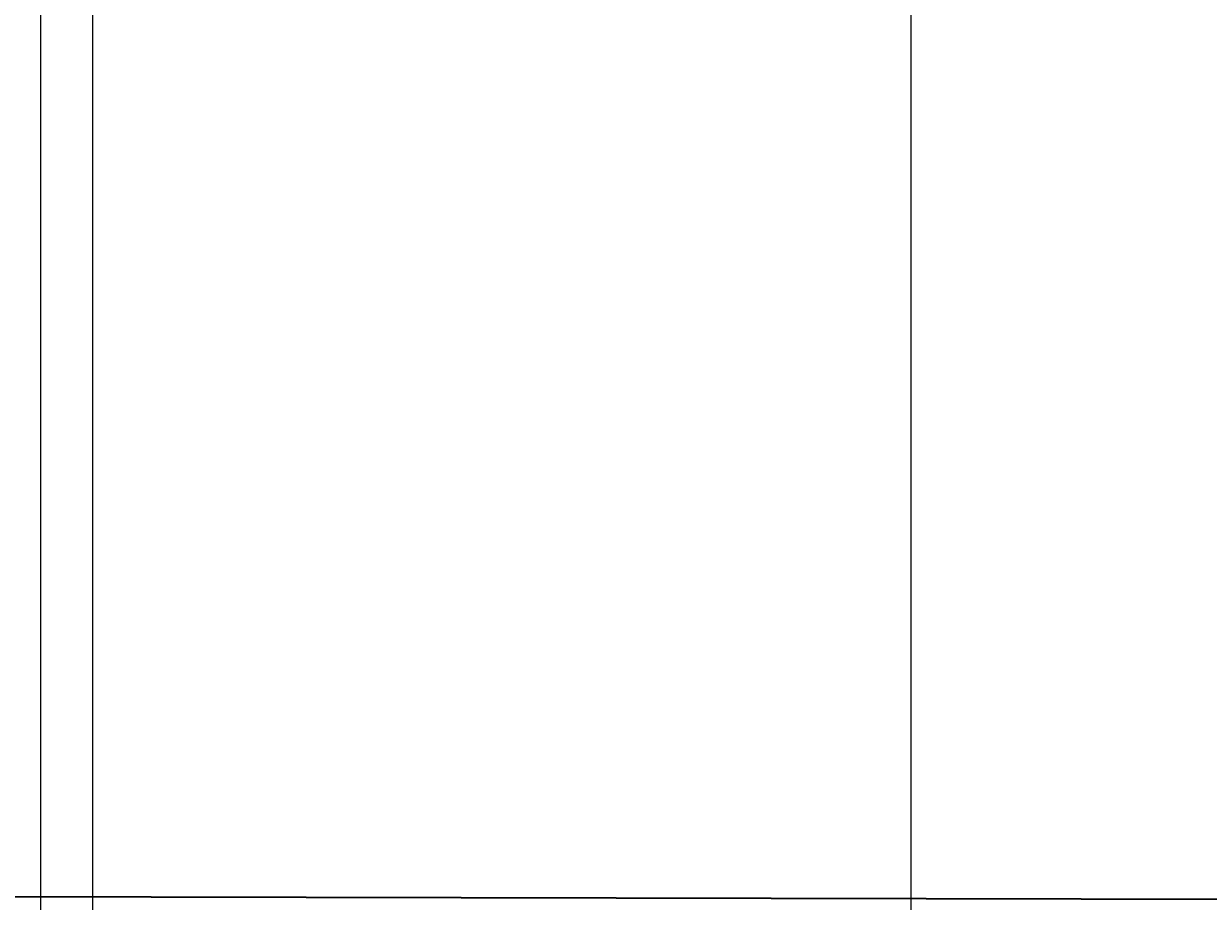
# Model space of a CAD drawing. Units: inches. Extents: x 27 to 200, y -50 to 102.
# Tile 21 of 26: x 145 to 172, y 19 to 39. Entities that reach past the tile are written whole.
import ezdxf

# ---------------------------------------------------------------- set-up
doc = ezdxf.new("R2010")
doc.units = ezdxf.units.IN
doc.header["$MEASUREMENT"] = 0
doc.layers.add('A-ANNO-DIMS', color=2, linetype='Continuous', lineweight=18)
doc.layers.add('A-ELEV', color=7, linetype='Continuous', lineweight=35)
doc.styles.get("Standard").update_dxf_attribs({"font": 'arial.ttf'})
doc.dimstyles.get("Standard").update_dxf_attribs({"dimtxt": 0.18, "dimasz": 0.18, "dimexe": 0.18, "dimexo": 0.0625, "dimgap": 0.09, "dimtad": 0, "dimtih": 1, "dimtoh": 1, "dimdec": 4, "dimzin": 0, "dimdsep": 46, "dimtxsty": 'Standard', "dimcen": 0.09, "dimadec": 0, "dimazin": 0, "dimtfac": 1, "dimtdec": 4, "dimtofl": 0, "dimtmove": 0, "dimatfit": 3, "dimfxl": 1, "dimtolj": 1, "dimtzin": 0, "dimarcsym": 0})

# ---------------------------------------------------------------- blocks, each defined once
blk = doc.blocks.new('*D48')
at = {"layer": 'A-ANNO-DIMS', "color": 0, "lineweight": -2, "transparency": 16777216}
for p, q in [((84.479, 44.926), (199.797, 44.926)), ((199.617, 44.746), (199.617, 14.26)), ((199.617, -16.589), (199.617, 13.897)), ((84.479, -16.769), (199.797, -16.769))]:
    blk.add_line(p, q, dxfattribs=at)
at = {"layer": 'A-ANNO-DIMS', "color": 0, "transparency": 16777216}
for points in [[(199.587, 44.746), (199.647, 44.746), (199.617, 44.926)], [(199.587, -16.589), (199.647, -16.589), (199.617, -16.769)]]:
    blk.add_solid(points, dxfattribs=at)
at = {"layer": 'Defpoints', "color": 0, "transparency": 16777216}
for p in [(84.417, 44.926), (199.617, 44.926), (84.417, -16.769)]:
    blk.add_point(p, dxfattribs=at)
at = {"layer": 'A-ANNO-DIMS', "color": 0, "transparency": 16777216, "insert": (199.617, 14.079), "char_height": 0.18, "attachment_point": 5}
blk.add_mtext('\\A1;61.7', dxfattribs=at)
blk = doc.blocks.new('*D51')
at = {"layer": 'A-ANNO-DIMS', "color": 0, "lineweight": -2, "transparency": 16777216}
for p, q in [((120.417, 45.561), (120.417, -25.149)), ((146.417, 45.561), (146.417, -25.149)), ((120.597, -24.969), (133.197, -24.969)), ((146.237, -24.969), (133.637, -24.969))]:
    blk.add_line(p, q, dxfattribs=at)
at = {"layer": 'A-ANNO-DIMS', "color": 0, "transparency": 16777216}
for points in [[(120.597, -24.939), (120.597, -24.999), (120.417, -24.969)], [(146.237, -24.939), (146.237, -24.999), (146.417, -24.969)]]:
    blk.add_solid(points, dxfattribs=at)
at = {"layer": 'Defpoints', "color": 0, "transparency": 16777216}
for p in [(120.417, 45.623), (146.417, 45.623), (146.417, -24.969)]:
    blk.add_point(p, dxfattribs=at)
at = {"layer": 'A-ANNO-DIMS', "color": 0, "transparency": 16777216, "insert": (133.417, -24.969), "char_height": 0.18, "attachment_point": 5}
blk.add_mtext('\\A1;26', dxfattribs=at)
blk = doc.blocks.new('*D64')
at = {"layer": 'A-ANNO-DIMS', "color": 0, "lineweight": -2, "transparency": 16777216}
for p, q in [((145.216, 13.517), (145.216, 102.306)), ((145.396, 102.126), (154.884, 102.126)), ((165.303, 102.126), (155.815, 102.126)), ((165.483, 13.517), (165.483, 102.306))]:
    blk.add_line(p, q, dxfattribs=at)
at = {"layer": 'A-ANNO-DIMS', "color": 0, "transparency": 16777216}
for points in [[(145.396, 102.156), (145.396, 102.096), (145.216, 102.126)], [(165.303, 102.156), (165.303, 102.096), (165.483, 102.126)]]:
    blk.add_solid(points, dxfattribs=at)
at = {"layer": 'Defpoints', "color": 0, "transparency": 16777216}
for p in [(165.483, 102.126), (145.216, 13.455), (165.483, 13.455)]:
    blk.add_point(p, dxfattribs=at)
at = {"layer": 'A-ANNO-DIMS', "color": 0, "transparency": 16777216, "insert": (155.35, 102.126), "char_height": 0.18, "attachment_point": 5}
blk.add_mtext('\\A1;20.267', dxfattribs=at)

msp = doc.modelspace()

# ---------------------------------------------------------------- linework, layer by layer
at = {"layer": 'A-ELEV'}
msp.add_line((191.4169, 19.002), (89.3118, 19.2307), dxfattribs=at)

# ---------------------------------------------------------------- dimensions: what is measured, and where the dimension line sits
at = {"layer": 'A-ANNO-DIMS'}
for base, p1, p2, override, picture, middle in [((165.4832, 102.1264), (145.216, 13.4548), (165.4832, 13.4548), {"dimdec": 3, "dimlfac": 1, "dimrnd": 0, "dimzin": 0, "dimdsep": 46, "dimlunit": 2}, '*D64', (155.3496, 102.1264)), ((146.4169, -24.9693), (120.4169, 45.6231), (146.4169, 45.6231), {"dimdec": 0, "dimlfac": 1, "dimrnd": 0, "dimzin": 0, "dimdsep": 46, "dimlunit": 2}, '*D51', (133.4169, -24.9693))]:
    dim = msp.add_linear_dim(base=base, p1=p1, p2=p2, dimstyle='Standard', override=override, dxfattribs=at)
    dim.commit()
    dim.dimension.update_dxf_attribs({"geometry": picture, "text_midpoint": middle})
dim = msp.add_linear_dim(base=(199.6169, 44.9264), p1=(84.4169, -16.7693), p2=(84.4169, 44.9264), angle=90, dimstyle='Standard', override={"dimdec": 1, "dimlfac": 1, "dimrnd": 0, "dimzin": 0, "dimdsep": 46, "dimlunit": 2}, dxfattribs=at)
dim.commit()
dim.dimension.update_dxf_attribs({"geometry": '*D48', "text_midpoint": (199.6169, 14.0786)})

doc.saveas('drawing.dxf')
